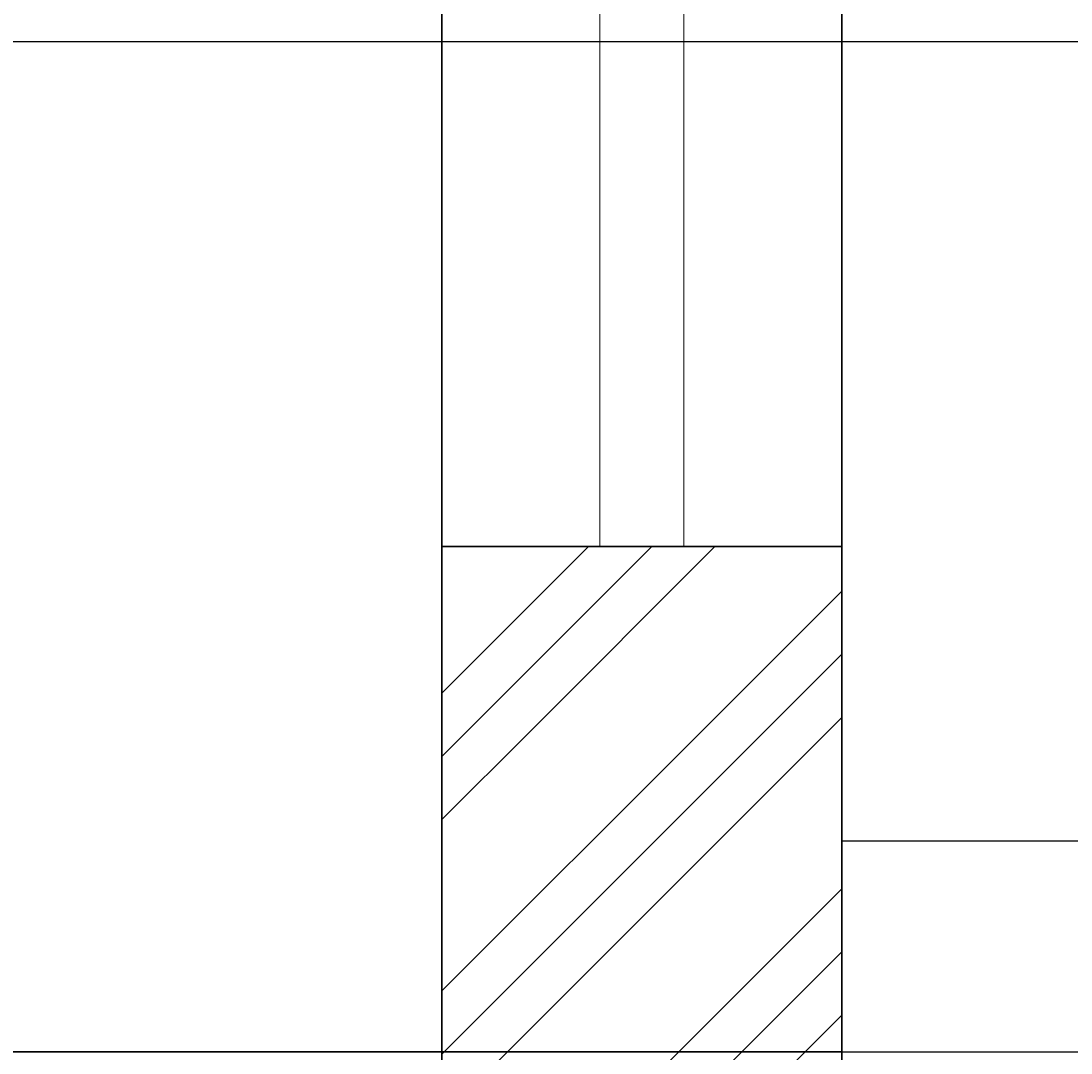
# Model space of a CAD drawing. Units: inches. Extents: x -128 to 854, y -395 to 398.
# Tile 17 of 61: x 279 to 329, y -298 to -249. Entities that reach past the tile are written whole.
import ezdxf

# ---------------------------------------------------------------- set-up
doc = ezdxf.new("R2010")
doc.units = ezdxf.units.IN
doc.header["$MEASUREMENT"] = 0
for name, color, linetype, lineweight in [('A-ANNO-DIMS', 2, 'Continuous', 18), ('A-FLOR-STRS', 7, 'Continuous', 25), ('A-GLAZ', 220, 'Continuous', 18), ('A-SECT', 220, 'Continuous', 35), ('A-SECT-PATT', 8, 'Continuous', 13), ('C-GRAD', 7, 'Continuous', 25), ('S-FNDN', 2, 'Continuous', 35)]:
    doc.layers.add(name, color=color, linetype=linetype, lineweight=lineweight)
doc.styles.get("Standard").update_dxf_attribs({"font": 'arial.ttf'})
doc.dimstyles.get("Standard").update_dxf_attribs({"dimtxt": 0.18, "dimasz": 0.18, "dimexe": 0.18, "dimexo": 0.0625, "dimgap": 0.09, "dimtad": 0, "dimtih": 1, "dimtoh": 1, "dimdec": 1, "dimzin": 0, "dimdsep": 46, "dimlunit": 4, "dimtxsty": 'Standard', "dimcen": 0.09, "dimclrd": 1, "dimclre": 2, "dimclrt": 6, "dimadec": 0, "dimazin": 0, "dimtfac": 1, "dimtdec": 1, "dimtofl": 0, "dimtmove": 0, "dimatfit": 3, "dimfxl": 1, "dimtfill": 2, "dimtfillclr": 3, "dimtolj": 1, "dimtzin": 0, "dimarcsym": 0})
pattern_1 = [(45, (0, 0), (14.14214, -9e-16), [20]), (45, (3, 0), (14.14214, -9e-16), [20]), (45, (6, 0), (14.14214, -9e-16), [20])]

# ---------------------------------------------------------------- blocks, each defined once
blk = doc.blocks.new('ENTRY-STEPS-SECTION')
for p, q in [((12, 5), (12, 10)), ((12, 10), (24, 10)), ((0, 0), (0, 5)), ((0, 5), (12, 5)), ((24, 0), (0, 0))]:
    blk.add_line(p, q)
blk = doc.blocks.new('*D120')
at = {"layer": 'A-ANNO-DIMS', "color": 2, "lineweight": -2, "transparency": 16777216}
for p, q in [((317.902, -178.019), (389.719, -178.019)), ((337.902, -358.019), (389.719, -358.019))]:
    blk.add_line(p, q, dxfattribs=at)
at = {"layer": 'A-ANNO-DIMS', "color": 1, "lineweight": -2, "transparency": 16777216}
for p, q in [((389.539, -178.199), (389.539, -267.837)), ((389.539, -357.839), (389.539, -268.201))]:
    blk.add_line(p, q, dxfattribs=at)
at = {"layer": 'A-ANNO-DIMS', "color": 1, "transparency": 16777216}
for points in [[(389.509, -178.199), (389.569, -178.199), (389.539, -178.019)], [(389.509, -357.839), (389.569, -357.839), (389.539, -358.019)]]:
    blk.add_solid(points, dxfattribs=at)
at = {"layer": 'Defpoints', "color": 0, "transparency": 16777216}
for p in [(317.839, -178.019), (337.839, -358.019), (389.539, -358.019)]:
    blk.add_point(p, dxfattribs=at)
at = {"layer": 'A-ANNO-DIMS', "color": 6, "transparency": 16777216, "insert": (389.539, -268.019), "char_height": 0.18, "attachment_point": 5, "bg_fill": 1, "box_fill_scale": 1.25, "bg_fill_color": 3, "bg_fill_transparency": 0}
blk.add_mtext('\\A1;15\'-0"', dxfattribs=at)
blk = doc.blocks.new('*D127')
at = {"layer": 'A-ANNO-DIMS', "color": 2, "lineweight": -2, "transparency": 16777216}
for p, q in [((260.902, -202.019), (389.719, -202.019)), ((317.902, -298.019), (389.719, -298.019))]:
    blk.add_line(p, q, dxfattribs=at)
at = {"layer": 'A-ANNO-DIMS', "color": 1, "lineweight": -2, "transparency": 16777216}
for p, q in [((389.539, -202.199), (389.539, -249.837)), ((389.539, -297.839), (389.539, -250.201))]:
    blk.add_line(p, q, dxfattribs=at)
at = {"layer": 'A-ANNO-DIMS', "color": 1, "transparency": 16777216}
for points in [[(389.509, -202.199), (389.569, -202.199), (389.539, -202.019)], [(389.509, -297.839), (389.569, -297.839), (389.539, -298.019)]]:
    blk.add_solid(points, dxfattribs=at)
at = {"layer": 'Defpoints', "color": 0, "transparency": 16777216}
for p in [(260.839, -202.019), (389.539, -202.019), (317.839, -298.019)]:
    blk.add_point(p, dxfattribs=at)
at = {"layer": 'A-ANNO-DIMS', "color": 6, "transparency": 16777216, "insert": (389.539, -250.019), "char_height": 0.18, "attachment_point": 5, "bg_fill": 1, "box_fill_scale": 1.25, "bg_fill_color": 3, "bg_fill_transparency": 0}
blk.add_mtext('\\A1;8\'-0"', dxfattribs=at)
blk = doc.blocks.new('*D132')
at = {"layer": 'A-ANNO-DIMS', "color": 2, "lineweight": -2, "transparency": 16777216}
for p, q in [((198.902, -250.019), (389.719, -250.019)), ((160.902, -298.019), (389.719, -298.019))]:
    blk.add_line(p, q, dxfattribs=at)
at = {"layer": 'A-ANNO-DIMS', "color": 1, "lineweight": -2, "transparency": 16777216}
for p, q in [((389.539, -250.199), (389.539, -273.837)), ((389.539, -297.839), (389.539, -274.201))]:
    blk.add_line(p, q, dxfattribs=at)
at = {"layer": 'A-ANNO-DIMS', "color": 1, "transparency": 16777216}
for points in [[(389.509, -250.199), (389.569, -250.199), (389.539, -250.019)], [(389.509, -297.839), (389.569, -297.839), (389.539, -298.019)]]:
    blk.add_solid(points, dxfattribs=at)
at = {"layer": 'Defpoints', "color": 0, "transparency": 16777216}
for p in [(198.839, -250.019), (389.539, -250.019), (160.839, -298.019)]:
    blk.add_point(p, dxfattribs=at)
at = {"layer": 'A-ANNO-DIMS', "color": 6, "transparency": 16777216, "insert": (389.539, -274.019), "char_height": 0.18, "attachment_point": 5, "bg_fill": 1, "box_fill_scale": 1.25, "bg_fill_color": 3, "bg_fill_transparency": 0}
blk.add_mtext('\\A1;4\'-0"', dxfattribs=at)

msp = doc.modelspace()

# ---------------------------------------------------------------- hatches: boundary and pattern name
at = {"layer": 'A-SECT-PATT'}
h = msp.add_hatch(dxfattribs=at)
h.set_pattern_fill('GOST_GROUND', color=256)
h.set_pattern_definition(pattern_1)
h.paths.add_polyline_path([(-37.161, -178.019), (-56.161, -178.019), (-56.161, -202.019), (-37.161, -202.019)])
h.paths.add_polyline_path([(160.839, -178.019), (141.839, -178.019), (141.839, -202.019), (160.839, -202.019)])
h.paths.add_polyline_path([(160.839, -207.019), (141.839, -207.019), (141.839, -226.019), (160.839, -226.019)])
h.paths.add_polyline_path([(317.839, -178.019), (298.839, -178.019), (298.839, -202.019), (317.839, -202.019)])
h.paths.add_polyline_path([(317.839, -207.019), (298.839, -207.019), (298.839, -226.019), (317.839, -226.019)])
h.paths.add_polyline_path([(317.839, -274.019), (298.839, -274.019), (298.839, -298.019), (303.839, -298.019), (312.839, -298.019), (317.839, -298.019)])
h = msp.add_hatch(dxfattribs=at)
h.set_pattern_fill('GOST_GROUND', color=256)
h.set_pattern_definition(pattern_1)
h.paths.add_polyline_path([(-27.161, -322.019), (-37.161, -322.019), (-37.161, -298.019), (-56.161, -298.019), (-56.161, -322.019), (-66.161, -322.019), (-66.161, -346.019), (-27.161, -346.019)])
h.paths.add_polyline_path([(170.839, -322.019), (160.839, -322.019), (160.839, -298.019), (155.839, -298.019), (141.839, -298.019), (141.839, -322.019), (131.839, -322.019), (131.839, -346.019), (170.839, -346.019)])
h.paths.add_polyline_path([(327.839, -322.019), (317.839, -322.019), (317.839, -298.019), (312.839, -298.019), (298.839, -298.019), (298.839, -322.019), (288.839, -322.019), (288.839, -346.019), (327.839, -346.019)])
h.paths.add_polyline_path([(-37.161, -274.019), (-56.161, -274.019), (-56.161, -298.019), (-37.161, -298.019)])
h.paths.add_polyline_path([(-37.161, -207.019), (-56.161, -207.019), (-56.161, -226.019), (-37.161, -226.019)])
h.paths.add_polyline_path([(160.839, -274.019), (141.839, -274.019), (141.839, -298.019), (155.839, -298.019), (160.839, -298.019)])

# ---------------------------------------------------------------- linework, layer by layer
at = {"layer": 'A-GLAZ'}
for p, q in [((306.339, -226.019), (306.339, -274.019)), ((310.339, -226.019), (310.339, -274.019))]:
    msp.add_line(p, q, dxfattribs=at)
at = {"layer": 'A-SECT'}
for p, q in [((298.839, -298.019), (298.839, -178.019)), ((317.839, -298.019), (317.839, -178.019)), ((298.839, -274.019), (317.839, -274.019)), ((-56.161, -298.019), (312.839, -298.019)), ((303.839, -298.019), (298.839, -298.019)), ((312.839, -298.019), (317.839, -298.019))]:
    msp.add_line(p, q, dxfattribs=at)
at = {"layer": 'C-GRAD'}
msp.add_line((317.839, -298.019), (365.839, -298.019), dxfattribs=at)
at = {"layer": 'S-FNDN'}
for p, q in [((303.839, -298.019), (298.839, -298.019)), ((298.839, -298.019), (298.839, -322.019)), ((312.839, -298.019), (317.839, -298.019)), ((317.839, -298.019), (317.839, -322.019))]:
    msp.add_line(p, q, dxfattribs=at)

# ---------------------------------------------------------------- block references
at = {"layer": 'A-FLOR-STRS', "extrusion": (0, 0, -1), "zscale": -1}
msp.add_blockref('ENTRY-STEPS-SECTION', (-341.839, -298.019), dxfattribs=at)

# ---------------------------------------------------------------- dimensions: what is measured, and where the dimension line sits
at = {"layer": 'A-ANNO-DIMS'}
for base, p1, p2, picture, middle in [((389.539, -358.019), (317.839, -178.019), (337.839, -358.019), '*D120', (389.539, -268.019)), ((389.539, -202.019), (317.839, -298.019), (260.839, -202.019), '*D127', (389.539, -250.019)), ((389.539, -250.019), (160.839, -298.019), (198.839, -250.019), '*D132', (389.539, -274.019))]:
    dim = msp.add_linear_dim(base=base, p1=p1, p2=p2, angle=90, dimstyle='Standard', override={"dimdec": 1, "dimlfac": 1, "dimrnd": 0, "dimzin": 1, "dimdsep": 46, "dimlunit": 4, "dimfrac": 2}, dxfattribs=at)
    dim.commit()
    dim.dimension.update_dxf_attribs({"geometry": picture, "text_midpoint": middle})

doc.saveas('drawing.dxf')
